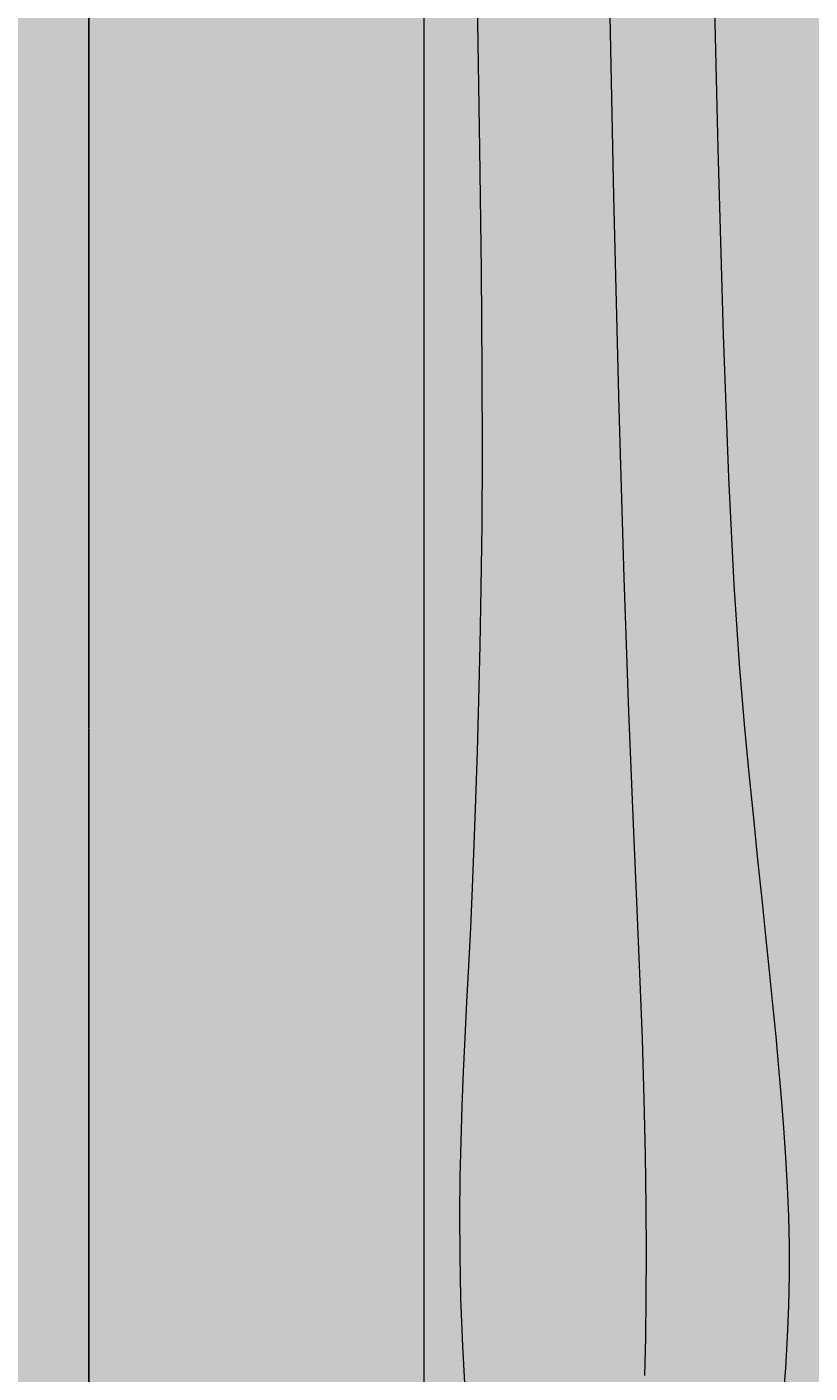
# Model space of a CAD drawing. Units: millimetres. Extents: x -229 to 16545, y -10488 to 4272.
# Tile 16 of 29: x 11804 to 12216, y -3417 to -2708. Entities that reach past the tile are written whole.
import ezdxf

# ---------------------------------------------------------------- set-up
doc = ezdxf.new("R2010")
doc.units = ezdxf.units.MM
for name, color, linetype, lineweight in [('A-ANNO-DIMS', 2, 'Continuous', 18), ('A-FURN', 8, 'Continuous', 18), ('A-FURN-PATT', 252, 'Continuous', 13)]:
    doc.layers.add(name, color=color, linetype=linetype, lineweight=lineweight)
doc.layers.add('A-FLOR-PATT', color=254, linetype='Continuous', lineweight=13, true_color=0xfeeab9)
doc.styles.get("Standard").update_dxf_attribs({"font": 'arial.ttf'})
doc.dimstyles.get("Standard").update_dxf_attribs({"dimtxt": 0.18, "dimasz": 0.18, "dimexe": 0.18, "dimexo": 0.0625, "dimgap": 0.09, "dimtad": 0, "dimtih": 1, "dimtoh": 1, "dimdec": 4, "dimzin": 0, "dimdsep": 46, "dimtxsty": 'Standard', "dimcen": 0.09, "dimadec": 0, "dimazin": 0, "dimtfac": 1, "dimtdec": 4, "dimtofl": 0, "dimtmove": 0, "dimatfit": 3, "dimfxl": 1, "dimtolj": 1, "dimtzin": 0, "dimarcsym": 0})

# ---------------------------------------------------------------- blocks, each defined once
blk = doc.blocks.new('Table - Rectangular Woodgrain 60 x 30 in.')
blk.add_line((0, -30), (60, -30))
for points in [[(8.0098, -22.2501), (14.4094, -22.1011), (19.4168, -21.9535), (23.25, -21.8083), (26.1269, -21.6663), (28.2656, -21.5281), (29.884, -21.3947), (31.2, -21.2667), (32.3967, -21.1448), (33.5172, -21.0292), (34.5697, -20.9198), (35.5625, -20.8167), (36.5037, -20.7198), (37.4015, -20.6292), (38.2642, -20.5448), (39.1, -20.4667), (39.9164, -20.3951), (40.7187, -20.3313), (41.5117, -20.2768), (42.3, -20.2333), (43.0883, -20.2024), (43.8812, -20.1854), (44.6836, -20.1841), (45.5, -20.2), (46.3328, -20.234), (47.1747, -20.2844), (48.0163, -20.3488)], [(8.6355, -25.0504), (15.7026, -24.9031), (21.4049, -24.7606), (25.9458, -24.625), (29.529, -24.4988), (32.3578, -24.3844), (34.6359, -24.284), (36.5667, -24.2), (38.3213, -24.1341), (39.9417, -24.0854), (41.437, -24.0523), (42.8167, -24.0333), (44.0901, -24.0268), (45.2667, -24.0313), (46.3557, -24.0451), (47.3667, -24.0667)], [(10.45, -28.5698), (14.407, -28.5012), (17.675, -28.4584), (20.3711, -28.4374), (22.6125, -28.4344), (24.5164, -28.4455), (26.2, -28.4667), (27.762, -28.4947), (29.2276, -28.5281), (30.6033, -28.5663), (31.8958, -28.6084), (33.1118, -28.6535), (34.2578, -28.7011), (35.3405, -28.7501), (36.3666, -28.8), (37.3443, -28.8497), (38.288, -28.8974), (39.2137, -28.9412), (40.1375, -28.9792), (41.0753, -29.0093), (42.0432, -29.0297), (43.0572, -29.0384), (44.1333, -29.0333), (45.2936, -29.0114), (46.5843, -28.9641), (48.0579, -28.8816)]]:
    blk.add_lwpolyline(points)
blk = doc.blocks.new('*D41')
at = {"layer": 'A-ANNO-DIMS', "color": 0, "lineweight": -2, "transparency": 16777216}
for p, q in [((12012.63, -2489.42), (11836.03, -2489.42)), ((11836.21, -2489.6), (11836.21, -3077.54)), ((11836.21, -3665.84), (11836.21, -3077.9)), ((12012.63, -3666.02), (11836.03, -3666.02))]:
    blk.add_line(p, q, dxfattribs=at)
at = {"layer": 'A-ANNO-DIMS', "color": 0, "transparency": 16777216}
for points in [[(11836.18, -2489.6), (11836.24, -2489.6), (11836.21, -2489.42)], [(11836.18, -3665.84), (11836.24, -3665.84), (11836.21, -3666.02)]]:
    blk.add_solid(points, dxfattribs=at)
at = {"layer": 'Defpoints', "color": 0, "transparency": 16777216}
for p in [(12012.7, -2489.42), (11836.21, -3666.02), (12012.7, -3666.02)]:
    blk.add_point(p, dxfattribs=at)
at = {"layer": 'A-ANNO-DIMS', "color": 0, "transparency": 16777216, "insert": (11836.21, -3077.72), "char_height": 0.18, "attachment_point": 5}
blk.add_mtext('\\A1;LOW TABLE 1177', dxfattribs=at)
blk = doc.blocks.new('*D101')
at = {"layer": 'A-ANNO-DIMS', "color": 0, "lineweight": -2, "transparency": 16777216}
for p, q in [((10907.81, -3049.71), (10907.99, -3049.71)), ((10907.9, -3049.8), (10907.9, -3049.62)), ((15176.85, -3049.71), (13576.18, -3049.71))]:
    blk.add_line(p, q, dxfattribs=at)
at = {"layer": 'A-ANNO-DIMS', "color": 0, "transparency": 16777216}
blk.add_solid([(13576.18, -3049.68), (13576.18, -3049.74), (13576, -3049.71)], dxfattribs=at)
at = {"layer": 'Defpoints', "color": 0, "transparency": 16777216}
for p in [(10907.9, -3049.71), (13576, -3049.71)]:
    blk.add_point(p, dxfattribs=at)
at = {"layer": 'A-ANNO-DIMS', "color": 0, "transparency": 16777216, "insert": (15177.3, -3049.71), "char_height": 0.18, "attachment_point": 5}
blk.add_mtext('\\A1;R2668', dxfattribs=at)
blk = doc.blocks.new('*D102')
at = {"layer": 'A-ANNO-DIMS', "color": 0, "lineweight": -2, "transparency": 16777216}
for p, q in [((11192.83, -3049.71), (11193.01, -3049.71)), ((11192.92, -3049.8), (11192.92, -3049.62)), ((15217.18, -3049.71), (13708.26, -3049.71))]:
    blk.add_line(p, q, dxfattribs=at)
at = {"layer": 'A-ANNO-DIMS', "color": 0, "transparency": 16777216}
blk.add_solid([(13708.26, -3049.68), (13708.26, -3049.74), (13708.08, -3049.71)], dxfattribs=at)
at = {"layer": 'Defpoints', "color": 0, "transparency": 16777216}
for p in [(11192.92, -3049.71), (13708.08, -3049.71)]:
    blk.add_point(p, dxfattribs=at)
at = {"layer": 'A-ANNO-DIMS', "color": 0, "transparency": 16777216, "insert": (15217.62, -3049.71), "char_height": 0.18, "attachment_point": 5}
blk.add_mtext('\\A1;R2515', dxfattribs=at)

msp = doc.modelspace()

# ---------------------------------------------------------------- hatches: boundary and pattern name
at = {"layer": 'A-FLOR-PATT', "transparency": 33554592}
h = msp.add_hatch(color=256, dxfattribs=at)
h.dxf.hatch_style = 1
h.paths.add_polyline_path([(7975.933, -5325.772), (7943.121, -5325.772), (7943.121, -4576.49, 0.4014527), (7225.933, -5325.772, 0.4014527), (6508.746, -4576.49), (6508.746, -5325.772), (6475.933, -5325.772), (6475.933, -5438.272), (5975.933, -5438.272), (5975.933, -7267.724), (5975.933, -7438.272), (6478.619, -7438.272), (6463.448, -7355.919), (6464.88, -7356.837), (6463.849, -7358.097), (6478.619, -7438.272), (6610.327, -7438.272), (6632.656, -7409.564), (6632.525, -7406.967), (6634.208, -7407.569), (6619.273, -7426.77), (6654.466, -7438.272), (7610.517, -7438.272), (7607.41, -7421.409), (7608.842, -7422.327), (7607.812, -7423.587), (7610.517, -7438.272), (7975.933, -7438.272)])
h.paths.add_polyline_path([(13785.933, -1208.272), (9555.933, -1208.272), (9555.933, -961.785), (9705.933, -961.785), (9705.933, -918.035), (10704.976, -918.035, 0.4014527), (9705.933, 38.215), (9555.933, 38.215), (9555.933, 2021.728), (5975.933, 2021.728), (5975.933, 755.492), (5745.933, 755.492), (5745.933, 1427.266), (2918.813, 1427.266), (2918.813, -492.942), (5013.319, -492.942), (5013.319, -978.272), (5745.933, -978.272), (5745.933, -397.513), (5975.933, -397.513), (5975.933, -1208.272), (4560.933, -1208.272), (4560.933, -1265.772), (4448.433, -1265.772), (4448.433, -1298.585), (4445.933, -1298.585), (3699.151, -1298.585, 0.4014527), (4448.433, -2015.772), (4560.933, -2015.772), (4560.933, -2384.177), (5745.933, -2384.177), (5799.402, -2384.177), (5799.402, -4518.272), (5975.933, -4518.272), (5975.933, -5208.272), (6475.933, -5208.272), (6475.933, -4575.772), (6508.746, -4575.772), (6508.746, -4576.49, -0.3564726), (7216.672, -5208.272), (7235.194, -5208.272, -0.3564726), (7943.121, -4576.49), (7943.121, -4575.772), (7975.933, -4575.772), (7975.933, -5208.272), (11176.247, -5208.272), (11159.44, -5191.465), (10520.768, -5191.465), (10520.768, -4888.936), (10571.19, -4888.936), (10571.19, -4872.129), (10772.876, -4872.129), (10772.876, -4888.936), (10789.683, -4888.936), (10789.683, -4872.129), (10991.368, -4872.129), (10991.368, -4888.936), (11041.79, -4888.936), (11041.79, -4872.129), (11058.597, -4872.129, -0.0909091), (11428.354, -4872.129), (11445.162, -4872.129), (11445.162, -4888.936), (11529.197, -4888.936), (11529.197, -5191.465), (11327.512, -5191.465), (11310.704, -5208.272), (13785.933, -5208.272)])
h.paths.add_polyline_path([(11047.216, -1630.944, -1), (11402.816, -1630.944, -1)], flags=16)
h.paths.add_polyline_path([(11148.816, -1630.944), (11225.016, -1554.744), (11301.216, -1630.944), (11225.016, -1707.144)], flags=0)
h.paths.add_polyline_path([(11199.616, -1630.944, -1), (11250.416, -1630.944, -1)], flags=0)
h.paths.add_polyline_path([(11588.751, -2096.259), (11588.751, -1543.254, -0.266667), (12864.918, -1543.254), (12864.918, -2096.259), (12737.302, -2096.259), (12737.302, -2063.121), (11716.368, -2063.121), (11716.368, -2096.259)], flags=16)
h.paths.add_polyline_path([(12012.696, -2489.42), (12600.997, -2489.42), (12600.997, -3666.022), (12012.696, -3666.022)], flags=16)
h.paths.add_polyline_path([(12176.41, -3599.403), (12174.938, -3609.076), (12173.789, -3618.819), (12173.09, -3628.559), (12172.973, -3638.221), (12173.89, -3652.852), (12175.008, -3657.025), (12172.909, -3643.473), (12173.142, -3624.297), (12175.386, -3605.273)], flags=0)
h.paths.add_polyline_path([(8026.289, -286.944), (7737.703, -287.19), (7734.87, -269.156), (8029.092, -268.905)], flags=16)
h.paths.add_polyline_path([(7733.453, -260.139), (7710.784, -115.865), (7557.191, -115.996), (7556.999, 109.744), (7412.687, 132.166), (7412.433, 429.206), (7556.707, 451.876), (7556.568, 614.769), (7412.256, 637.19), (7412.003, 934.231), (7556.276, 956.9), (7556.084, 1182.639), (7709.677, 1182.77), (7732.099, 1327.082), (8029.14, 1327.335), (8051.808, 1183.062), (8205.401, 1183.192), (8205.594, 957.454), (8349.906, 935.031), (8350.159, 637.99), (8205.885, 615.322), (8206.024, 452.43), (8350.336, 430.006), (8350.59, 132.965), (8206.316, 110.298), (8206.509, -115.442), (8052.916, -115.573), (8030.493, -259.885)], flags=16)
h.paths.add_polyline_path([(12261.416, -3475.554), (12262.632, -3486.776), (12264.032, -3497.007), (12265.554, -3506.365), (12267.136, -3514.968), (12268.719, -3522.935), (12271.304, -3535.59), (12273.606, -3548.078), (12275.271, -3561.064), (12275.93, -3574.938), (12275.325, -3590.3), (12273.425, -3607.964), (12270.795, -3625.658), (12268.066, -3641.063), (12266.318, -3649.679), (12265.456, -3653.626), (12263.984, -3659.846), (12264.032, -3659.566), (12264.342, -3658.241), (12264.807, -3656.37), (12265.456, -3653.626), (12266.318, -3649.679), (12267.409, -3644.302), (12268.668, -3637.664), (12270.019, -3630.037), (12271.384, -3621.695), (12272.69, -3612.908), (12273.857, -3603.948), (12274.81, -3595.088), (12275.47, -3586.601), (12275.782, -3578.689), (12275.757, -3571.292), (12275.423, -3564.275), (12274.816, -3557.512), (12273.964, -3550.872), (12272.896, -3544.224), (12271.645, -3537.439), (12270.24, -3530.385), (12267.543, -3517.181), (12264.612, -3501.247), (12261.849, -3481.059)], flags=0)
h.paths.add_polyline_path([(12332.136, -3408.03), (12333.483, -3416.79), (12335.077, -3424.54), (12336.915, -3431.355), (12338.991, -3437.32), (12341.266, -3442.55), (12343.694, -3447.166), (12346.229, -3451.292), (12348.826, -3455.051), (12351.438, -3458.563), (12357.476, -3466.491), (12363.61, -3476.575), (12368.309, -3489.762), (12369.929, -3503.427), (12369.842, -3516.511), (12368.43, -3530.867), (12365.816, -3545.835), (12362.382, -3559.786), (12360.968, -3564.487), (12363.063, -3557.021), (12364.898, -3549.566), (12366.473, -3542.077), (12367.773, -3534.631), (12368.781, -3527.301), (12369.483, -3520.162), (12369.863, -3513.291), (12369.906, -3506.759), (12369.599, -3500.643), (12368.93, -3494.999), (12367.924, -3489.796), (12366.61, -3484.994), (12365.024, -3480.542), (12363.19, -3476.399), (12361.141, -3472.516), (12358.909, -3468.847), (12356.525, -3465.347), (12354.02, -3461.954), (12351.438, -3458.563), (12345.462, -3450.529), (12339.923, -3439.996), (12335.85, -3428.296), (12332.68, -3412.888)], flags=0)
h.paths.add_polyline_path([(12385.287, -3334.612), (12384.977, -3342.409), (12385.02, -3349.196), (12385.4, -3355.066), (12386.104, -3360.105), (12387.112, -3364.41), (12388.412, -3368.071), (12389.987, -3371.181), (12391.823, -3373.832), (12393.919, -3376.097), (12396.337, -3377.978), (12399.153, -3379.462), (12402.445, -3380.531), (12406.289, -3381.172), (12410.758, -3381.371), (12415.935, -3381.106), (12421.893, -3380.368), (12428.658, -3379.159), (12436.069, -3377.55), (12443.907, -3375.635), (12451.961, -3373.505), (12460.015, -3371.254), (12467.853, -3368.971), (12475.263, -3366.749), (12482.029, -3364.68), (12491.877, -3361.657), (12497.701, -3360.107), (12501.639, -3359.288), (12510.135, -3358.326), (12519.662, -3365.412), (12524.243, -3378.911), (12523.764, -3390.7), (12520.746, -3401.577), (12514.248, -3415.634), (12511.518, -3420.418), (12515.856, -3412.154), (12519.153, -3405.024), (12521.516, -3398.804), (12523.049, -3393.276), (12523.865, -3388.212), (12524.059, -3383.441), (12523.7, -3378.958), (12522.853, -3374.815), (12521.576, -3371.054), (12519.931, -3367.722), (12517.982, -3364.865), (12515.786, -3362.529), (12513.405, -3360.758), (12510.877, -3359.588), (12508.136, -3358.982), (12505.086, -3358.897), (12501.639, -3359.288), (12497.701, -3360.107), (12493.183, -3361.309), (12487.988, -3362.851), (12476.403, -3366.408), (12463.335, -3370.326), (12447.372, -3374.788), (12431.759, -3378.604), (12418.504, -3380.974), (12405.811, -3381.624), (12394.725, -3378.025), (12388.039, -3368.367), (12385.583, -3357.877), (12384.826, -3346.204), (12385.428, -3331.059), (12385.953, -3325.719)], flags=0)
h.paths.add_polyline_path([(7880.016, 1173.969), (7880.373, 1175.495), (7880.433, 1175.851), (7879.484, 1171.818)], flags=0)
h.paths.add_polyline_path([(7802.33, 874.962), (7800.771, 885.032), (7798.932, 893.941), (7796.811, 901.774), (7794.419, 908.63), (7791.798, 914.639), (7789.002, 919.945), (7786.083, 924.686), (7783.093, 929.005), (7780.087, 933.043), (7774.996, 939.717), (7768.406, 949.37), (7762.174, 963.427), (7759.342, 978.002), (7758.629, 991.888), (7759.492, 1007.928), (7761.801, 1025.496), (7765.392, 1044.035), (7766.625, 1049.048), (7764.522, 1039.543), (7762.719, 1030.232), (7761.232, 1021.168), (7760.08, 1012.405), (7759.28, 1003.994), (7758.849, 995.988), (7758.806, 988.44), (7759.167, 981.404), (7759.942, 974.914), (7761.104, 968.936), (7762.617, 963.414), (7764.448, 958.299), (7766.559, 953.535), (7768.918, 949.073), (7771.487, 944.856), (7774.232, 940.835), (7777.115, 936.938), (7782.377, 930.041), (7787.845, 922.139), (7793.348, 911.698), (7798.042, 898.247), (7801.702, 880.527)], flags=0)
h.paths.add_polyline_path([(12519.068, -3228.534), (12519.615, -3236.235), (12520.529, -3242.343), (12521.78, -3247.103), (12523.337, -3250.758), (12525.171, -3253.556), (12527.248, -3255.709), (12529.522, -3257.296), (12531.95, -3258.361), (12534.486, -3258.949), (12537.082, -3259.11), (12539.694, -3258.888), (12542.277, -3258.329), (12544.781, -3257.478), (12547.173, -3256.388), (12549.46, -3255.129), (12550.455, -3254.517), (12555.825, -3251.109), (12557.835, -3249.942), (12565.181, -3246.404), (12574.565, -3253.032), (12576.931, -3265.022), (12576.627, -3277.425), (12575.416, -3290.819), (12574.851, -3295.392), (12575.708, -3287.593), (12576.322, -3280.806), (12576.688, -3274.939), (12576.812, -3269.899), (12576.688, -3265.593), (12576.322, -3261.932), (12575.708, -3258.822), (12574.851, -3256.172), (12573.753, -3253.905), (12572.439, -3252.005), (12570.943, -3250.474), (12569.293, -3249.309), (12567.523, -3248.513), (12565.658, -3248.083), (12563.732, -3248.022), (12561.777, -3248.328), (12559.814, -3248.989), (12557.835, -3249.942), (12555.825, -3251.109), (12553.77, -3252.413), (12551.652, -3253.78), (12549.46, -3255.129), (12543.167, -3258.594), (12532.661, -3259.485), (12524.685, -3253.923), (12520.949, -3245.152), (12519.138, -3233.042)], flags=0)
h.paths.add_polyline_path([(7741.293, 790.501), (7741.641, 799.467), (7741.584, 807.269), (7741.141, 814.015), (7740.329, 819.809), (7739.165, 824.757), (7737.667, 828.966), (7735.853, 832.541), (7733.74, 835.586), (7731.348, 838.188), (7728.71, 840.348), (7725.861, 842.052), (7722.836, 843.28), (7719.671, 844.015), (7716.4, 844.237), (7713.06, 843.932), (7709.684, 843.081), (7706.304, 841.686), (7702.923, 839.834), (7699.543, 837.629), (7696.164, 835.178), (7692.784, 832.585), (7684.718, 826.315), (7675.609, 820.63), (7664.001, 817.274), (7654.105, 821.884), (7647.171, 832.02), (7644.191, 846.522), (7646.321, 860.288), (7647.49, 864.223), (7645.946, 857.865), (7645.046, 852.044), (7644.827, 846.557), (7645.243, 841.404), (7646.221, 836.642), (7647.693, 832.318), (7649.587, 828.489), (7651.832, 825.206), (7654.359, 822.523), (7657.097, 820.49), (7659.984, 819.145), (7662.993, 818.452), (7666.108, 818.357), (7669.311, 818.809), (7672.583, 819.755), (7675.908, 821.139), (7679.268, 822.913), (7682.645, 825.021), (7686.025, 827.401), (7689.404, 829.958), (7692.784, 832.585), (7700.505, 838.509), (7709.871, 843.64), (7721.436, 844.698), (7733.277, 837.617), (7739.571, 825.214), (7741.557, 811.049), (7741.669, 795.575)], flags=0)
h.paths.add_polyline_path([(8377.641, 137.216), (8359.607, 134.382), (8359.356, 428.605), (8377.395, 425.802)], flags=16)
h.paths.add_polyline_path([(7650.715, 668.465), (7650.08, 677.319), (7649.023, 684.34), (7647.579, 689.811), (7645.785, 694.012), (7643.675, 697.228), (7641.286, 699.7), (7638.669, 701.521), (7635.876, 702.744), (7632.96, 703.419), (7629.974, 703.601), (7626.971, 703.344), (7624.004, 702.697), (7621.125, 701.717), (7618.375, 700.462), (7615.749, 699.013), (7614.561, 698.279), (7608.435, 694.382), (7606.125, 693.04), (7598.981, 689.594), (7589.669, 693.773), (7585.26, 702.856), (7584.221, 713.11), (7584.49, 724.584), (7585.863, 739.937), (7586.518, 745.277), (7585.539, 736.31), (7584.841, 728.507), (7584.424, 721.761), (7584.288, 715.966), (7584.433, 711.016), (7584.86, 706.807), (7585.567, 703.231), (7586.556, 700.186), (7587.821, 697.58), (7589.332, 695.397), (7591.053, 693.637), (7592.951, 692.3), (7594.989, 691.385), (7597.132, 690.895), (7599.346, 690.826), (7601.594, 691.18), (7603.851, 691.943), (7606.125, 693.04), (7608.435, 694.382), (7610.797, 695.885), (7613.229, 697.458), (7620.475, 701.929), (7632.001, 704.44), (7643.476, 699.417), (7648.536, 687.571), (7650.63, 673.661)], flags=0)
h.paths.add_polyline_path([(7385.628, 136.37), (7385.382, 424.956), (7403.416, 427.789), (7403.667, 133.567)], flags=16)
h.paths.add_polyline_path([(12993.884, -2257.186), (12959.588, -2257.186), (12959.588, -2125.099), (13531.966, -2125.099, -0.1904762), (13531.966, -3974.321), (12959.588, -3974.321), (12959.588, -3842.233), (12993.884, -3842.233)], flags=16)
h.paths.add_polyline_path([(13413.486, -3313.884), (13413.486, -2785.535), (13562.885, -2785.535, -0.0496282), (13562.885, -3313.884)], flags=0)
h.paths.add_polyline_path([(8377.21, 642.241), (8359.176, 639.407), (8358.925, 933.629), (8376.964, 930.826)], flags=16)
h.paths.add_polyline_path([(13086.058, -1864.83), (13086.058, -1449.84), (13501.048, -1449.84), (13501.048, -1864.83)], flags=16)
h.paths.add_polyline_path([(13305.814, -1862.197), (13302.103, -1859.624), (13298.088, -1857.068), (13293.799, -1854.536), (13289.262, -1852.031), (13284.504, -1849.559), (13279.554, -1847.125), (13274.439, -1844.735), (13269.17, -1842.389), (13263.701, -1840.081), (13257.97, -1837.797), (13251.914, -1835.525), (13245.472, -1833.252), (13238.582, -1830.968), (13231.18, -1828.66), (13223.206, -1826.315), (13209.182, -1822.458), (13204.584, -1821.48), (13217.962, -1824.773), (13235.072, -1829.804), (13248.777, -1834.349), (13260.829, -1838.869), (13274.479, -1844.63), (13289.675, -1852.101), (13302.553, -1859.704)], flags=0)
h.paths.add_polyline_path([(13428.104, -1820.994), (13419.007, -1818.141), (13409.95, -1815.4), (13400.766, -1812.747), (13391.271, -1810.151), (13376.087, -1806.251), (13370.618, -1805.019), (13386.304, -1808.794), (13405.087, -1813.928), (13423.014, -1819.354)], flags=0)
h.paths.add_polyline_path([(7385.197, 641.395), (7384.951, 929.98), (7402.986, 932.814), (7403.236, 638.592)], flags=16)
h.paths.add_polyline_path([(13262.537, -1725.526), (13253.246, -1724.74), (13244.516, -1724.117), (13235.94, -1723.625), (13223.267, -1723.062), (13217.598, -1722.912), (13231.966, -1723.397), (13248.733, -1724.359), (13266.899, -1725.895), (13272.802, -1726.502)], flags=0)
h.paths.add_polyline_path([(13191.893, -1641.137), (13208.675, -1640.506), (13214.057, -1640.258), (13197.763, -1640.936)], flags=0)
h.paths.add_polyline_path([(13097.524, -1608.457), (13114.284, -1609.031), (13120.126, -1609.105), (13103.045, -1608.71)], flags=0)
h.paths.add_polyline_path([(13465.328, -1521.577), (13473.906, -1517.015), (13481.761, -1511.636), (13492.562, -1502.076), (13495.327, -1497.933), (13485.818, -1508.858), (13470.208, -1519.547)], flags=0)
h.paths.add_polyline_path([(13175.015, -1500.891), (13184.046, -1501.807), (13192.721, -1502.52), (13201.114, -1503.034), (13209.273, -1503.351), (13217.244, -1503.476), (13225.078, -1503.41), (13232.821, -1503.16), (13240.524, -1502.728), (13248.233, -1502.117), (13255.993, -1501.322), (13263.825, -1500.293), (13271.746, -1498.974), (13279.775, -1497.305), (13287.928, -1495.229), (13296.222, -1492.688), (13304.675, -1489.622), (13313.304, -1485.975), (13322.089, -1481.727), (13330.859, -1477.028), (13339.408, -1472.063), (13347.526, -1467.02), (13355.006, -1462.087), (13364.86, -1455.202), (13367.224, -1453.299), (13358.544, -1459.754), (13343.348, -1469.775), (13326.143, -1479.767), (13309.023, -1488.045), (13292.249, -1494.129), (13276.009, -1498.264), (13260.299, -1500.88), (13244.401, -1502.51), (13228.945, -1503.378), (13213.316, -1503.508), (13197.047, -1502.876), (13180.088, -1501.481)], flags=0)
h.paths.add_polyline_path([(7733.501, 1336.101), (7736.303, 1354.14), (8024.889, 1354.386), (8027.723, 1336.352)], flags=16)
at = {"layer": 'A-FURN-PATT', "transparency": 33554569}
h = msp.add_hatch(color=256, dxfattribs=at)
h.dxf.hatch_style = 1
h.paths.add_polyline_path([(12600.997, -2489.42), (12553.933, -2489.42), (12553.58, -2583.852), (12552.584, -2666.503), (12551.036, -2738.644), (12549.03, -2801.547), (12546.656, -2856.483), (12544.004, -2904.723), (12541.171, -2947.542), (12538.245, -2986.207), (12535.313, -3021.787), (12532.444, -3054.526), (12529.695, -3084.461), (12527.132, -3111.629), (12524.814, -3136.073), (12522.802, -3157.826), (12521.157, -3176.928), (12519.941, -3193.42), (12519.202, -3207.371), (12518.921, -3218.994), (12519.068, -3228.534), (12519.615, -3236.235), (12520.529, -3242.343), (12521.78, -3247.103), (12523.337, -3250.758), (12525.171, -3253.556), (12527.248, -3255.709), (12529.522, -3257.296), (12531.95, -3258.361), (12534.486, -3258.949), (12537.082, -3259.11), (12539.694, -3258.888), (12542.277, -3258.329), (12544.781, -3257.478), (12547.173, -3256.388), (12549.46, -3255.129), (12551.652, -3253.78), (12559.563, -3248.675), (12566.794, -3247.543), (12572.687, -3251.706), (12575.978, -3258.498), (12576.872, -3267.431), (12576.627, -3277.425), (12575.708, -3287.593), (12574.851, -3295.392), (12573.749, -3304.309), (12572.419, -3314.522), (12570.874, -3326.221), (12569.131, -3339.597), (12567.203, -3354.842), (12565.107, -3372.146), (12562.857, -3391.705), (12560.469, -3413.705), (12557.959, -3438.275), (12555.343, -3465.264), (12552.633, -3494.46), (12549.848, -3525.645), (12547.001, -3558.61), (12544.106, -3593.137), (12541.184, -3629.012), (12538.245, -3666.022), (12600.997, -3666.022)])
h.paths.add_polyline_path([(12544.004, -2904.723), (12546.656, -2856.483), (12549.03, -2801.547), (12551.036, -2738.644), (12552.584, -2666.503), (12553.58, -2583.852), (12553.933, -2489.42), (12420.585, -2489.42), (12422.824, -2618.374), (12423.791, -2723.534), (12423.687, -2808.136), (12422.708, -2875.41), (12421.057, -2928.591), (12418.93, -2970.907), (12416.527, -3005.595), (12414.049, -3035.885), (12411.656, -3064.467), (12409.37, -3091.846), (12407.177, -3117.984), (12405.059, -3142.842), (12403.004, -3166.384), (12400.994, -3188.569), (12399.016, -3209.359), (12397.053, -3228.718), (12395.1, -3246.62), (12393.191, -3263.097), (12391.376, -3278.194), (12389.699, -3291.961), (12388.205, -3304.438), (12386.942, -3315.677), (12385.953, -3325.719), (12385.287, -3334.612), (12384.977, -3342.409), (12385.02, -3349.196), (12385.4, -3355.066), (12386.104, -3360.105), (12387.112, -3364.41), (12388.412, -3368.071), (12389.987, -3371.181), (12391.823, -3373.832), (12393.919, -3376.097), (12396.337, -3377.978), (12399.153, -3379.462), (12402.445, -3380.531), (12406.289, -3381.172), (12410.758, -3381.371), (12415.935, -3381.106), (12421.893, -3380.368), (12428.658, -3379.159), (12436.069, -3377.55), (12443.907, -3375.635), (12451.961, -3373.505), (12460.015, -3371.254), (12467.853, -3368.971), (12475.263, -3366.749), (12482.029, -3364.68), (12491.877, -3361.657), (12502.516, -3358.826), (12511.128, -3359.064), (12517.01, -3363.44), (12520.955, -3369.223), (12523.527, -3376.802), (12524.25, -3385.824), (12522.632, -3395.865), (12519.153, -3405.024), (12515.856, -3412.154), (12511.518, -3420.418), (12506.031, -3430.037), (12499.288, -3441.236), (12491.181, -3454.234), (12481.682, -3469.286), (12471.081, -3486.774), (12459.744, -3507.112), (12448.039, -3530.713), (12436.334, -3557.99), (12424.997, -3589.358), (12414.396, -3625.231), (12404.897, -3666.022), (12538.245, -3666.022), (12541.184, -3629.012), (12544.106, -3593.137), (12547.001, -3558.61), (12549.848, -3525.645), (12552.633, -3494.46), (12555.343, -3465.264), (12557.959, -3438.275), (12560.469, -3413.705), (12562.857, -3391.705), (12565.107, -3372.146), (12567.203, -3354.842), (12569.131, -3339.597), (12570.874, -3326.221), (12572.419, -3314.522), (12573.749, -3304.309), (12574.851, -3295.392), (12575.708, -3287.593), (12576.322, -3280.806), (12576.688, -3274.939), (12576.812, -3269.899), (12576.688, -3265.593), (12576.322, -3261.932), (12575.708, -3258.822), (12574.851, -3256.172), (12573.753, -3253.905), (12572.439, -3252.005), (12570.943, -3250.474), (12569.293, -3249.309), (12567.523, -3248.513), (12565.658, -3248.083), (12563.732, -3248.022), (12561.777, -3248.328), (12559.814, -3248.989), (12557.835, -3249.942), (12555.825, -3251.109), (12553.77, -3252.413), (12547.19, -3256.659), (12539.533, -3259.262), (12531.64, -3258.773), (12524.685, -3253.923), (12520.949, -3245.152), (12519.615, -3236.235), (12519.068, -3228.534), (12518.921, -3218.994), (12519.202, -3207.371), (12519.941, -3193.42), (12521.157, -3176.928), (12522.802, -3157.826), (12524.814, -3136.073), (12527.132, -3111.629), (12529.695, -3084.461), (12532.444, -3054.526), (12535.313, -3021.787), (12538.245, -2986.207), (12541.171, -2947.542)])
h.paths.add_polyline_path([(12418.93, -2970.907), (12421.057, -2928.591), (12422.708, -2875.41), (12423.687, -2808.136), (12423.791, -2723.534), (12422.824, -2618.374), (12420.585, -2489.42), (12349.989, -2489.42), (12347.396, -2591.092), (12345.433, -2678.094), (12343.99, -2752.122), (12342.962, -2814.864), (12342.239, -2868.017), (12341.715, -2913.271), (12341.284, -2952.323), (12340.837, -2986.86), (12340.288, -3018.358), (12339.633, -3047.386), (12338.883, -3074.301), (12338.06, -3099.455), (12337.173, -3123.199), (12336.242, -3145.885), (12335.279, -3167.868), (12334.301, -3189.498), (12333.326, -3211.038), (12332.381, -3232.395), (12331.496, -3253.384), (12330.706, -3273.821), (12330.037, -3293.523), (12329.52, -3312.306), (12329.188, -3329.984), (12329.071, -3346.378), (12329.194, -3361.343), (12329.561, -3374.915), (12330.175, -3387.169), (12331.032, -3398.18), (12332.136, -3408.03), (12333.483, -3416.79), (12335.077, -3424.54), (12336.915, -3431.355), (12338.991, -3437.32), (12341.266, -3442.55), (12343.694, -3447.166), (12346.229, -3451.292), (12348.826, -3455.051), (12351.438, -3458.563), (12357.476, -3466.491), (12362.356, -3474.514), (12365.989, -3482.725), (12368.611, -3492.308), (12369.929, -3503.427), (12369.863, -3513.291), (12369.483, -3520.162), (12368.781, -3527.301), (12367.773, -3534.631), (12366.473, -3542.077), (12364.898, -3549.566), (12363.063, -3557.021), (12360.968, -3564.487), (12358.568, -3572.468), (12355.799, -3581.585), (12352.603, -3592.463), (12348.916, -3605.723), (12344.678, -3621.988), (12339.827, -3641.88), (12334.301, -3666.022), (12404.897, -3666.022), (12414.396, -3625.231), (12424.997, -3589.358), (12436.334, -3557.99), (12448.039, -3530.713), (12459.744, -3507.112), (12471.081, -3486.774), (12481.682, -3469.286), (12491.181, -3454.234), (12499.288, -3441.236), (12506.031, -3430.037), (12511.518, -3420.418), (12515.856, -3412.154), (12519.153, -3405.024), (12521.516, -3398.804), (12523.049, -3393.276), (12523.865, -3388.212), (12524.059, -3383.441), (12523.7, -3378.958), (12522.853, -3374.815), (12521.576, -3371.054), (12519.931, -3367.722), (12517.982, -3364.865), (12515.786, -3362.529), (12513.405, -3360.758), (12510.877, -3359.588), (12508.136, -3358.982), (12505.086, -3358.897), (12501.639, -3359.288), (12497.701, -3360.107), (12493.183, -3361.309), (12487.988, -3362.851), (12476.403, -3366.408), (12463.335, -3370.326), (12451.961, -3373.505), (12439.372, -3376.834), (12424.661, -3380.026), (12412.995, -3381.47), (12402.039, -3380.984), (12393.748, -3376.613), (12389.022, -3369.787), (12386.442, -3362.522), (12385.041, -3352.492), (12384.977, -3342.409), (12385.287, -3334.612), (12385.953, -3325.719), (12386.942, -3315.677), (12388.205, -3304.438), (12389.699, -3291.961), (12391.376, -3278.194), (12393.191, -3263.097), (12395.1, -3246.62), (12397.053, -3228.718), (12399.016, -3209.359), (12400.994, -3188.569), (12403.004, -3166.384), (12405.059, -3142.842), (12407.177, -3117.984), (12409.37, -3091.846), (12411.656, -3064.467), (12414.049, -3035.885), (12416.527, -3005.595)])
h.paths.add_polyline_path([(12340.837, -2986.86), (12341.284, -2952.323), (12341.715, -2913.271), (12342.239, -2868.017), (12342.962, -2814.864), (12343.99, -2752.122), (12345.433, -2678.094), (12347.396, -2591.092), (12349.989, -2489.42), (12248.016, -2489.42), (12253.364, -2589.902), (12257.71, -2678.871), (12261.149, -2757.499), (12263.787, -2826.958), (12265.718, -2888.42), (12267.044, -2943.055), (12267.866, -2992.039), (12268.279, -3036.54), (12268.378, -3077.58), (12268.209, -3115.572), (12267.809, -3150.776), (12267.219, -3183.452), (12266.473, -3213.86), (12265.614, -3242.261), (12264.679, -3268.917), (12263.704, -3294.084), (12262.732, -3317.981), (12261.804, -3340.639), (12260.969, -3362.039), (12260.273, -3382.167), (12259.759, -3401.008), (12259.477, -3418.547), (12259.469, -3434.769), (12259.782, -3449.659), (12260.445, -3463.221), (12261.416, -3475.554), (12262.632, -3486.776), (12264.032, -3497.007), (12265.554, -3506.365), (12267.136, -3514.968), (12268.719, -3522.935), (12271.304, -3535.59), (12273.606, -3548.078), (12275.271, -3561.064), (12275.757, -3571.292), (12275.782, -3578.689), (12275.47, -3586.601), (12274.81, -3595.088), (12273.857, -3603.948), (12272.69, -3612.908), (12271.384, -3621.695), (12270.019, -3630.037), (12268.066, -3641.063), (12265.651, -3652.97), (12264.342, -3658.241), (12264.032, -3659.566), (12263.842, -3660.678), (12263.746, -3661.906), (12263.708, -3663.576), (12263.704, -3666.022), (12334.301, -3666.022), (12339.827, -3641.88), (12344.678, -3621.988), (12348.916, -3605.723), (12352.603, -3592.463), (12355.799, -3581.585), (12358.568, -3572.468), (12360.968, -3564.487), (12363.063, -3557.021), (12364.898, -3549.566), (12366.473, -3542.077), (12367.773, -3534.631), (12368.781, -3527.301), (12369.483, -3520.162), (12369.863, -3513.291), (12369.906, -3506.759), (12369.599, -3500.643), (12368.93, -3494.999), (12367.924, -3489.796), (12366.61, -3484.994), (12365.024, -3480.542), (12363.19, -3476.399), (12361.141, -3472.516), (12358.909, -3468.847), (12356.525, -3465.347), (12354.02, -3461.954), (12347.609, -3453.536), (12342.257, -3444.828), (12337.759, -3434.488), (12335.077, -3424.54), (12333.483, -3416.79), (12332.136, -3408.03), (12331.032, -3398.18), (12330.175, -3387.169), (12329.561, -3374.915), (12329.194, -3361.343), (12329.071, -3346.378), (12329.188, -3329.984), (12329.52, -3312.306), (12330.037, -3293.523), (12330.706, -3273.821), (12331.496, -3253.384), (12332.381, -3232.395), (12333.326, -3211.038), (12334.301, -3189.498), (12335.279, -3167.868), (12336.242, -3145.885), (12337.173, -3123.199), (12338.06, -3099.455), (12338.883, -3074.301), (12339.633, -3047.386), (12340.288, -3018.358)])
h.paths.add_polyline_path([(12267.866, -2992.039), (12267.044, -2943.055), (12265.718, -2888.42), (12263.787, -2826.958), (12261.149, -2757.499), (12257.71, -2678.871), (12253.364, -2589.902), (12248.016, -2489.42), (12161.732, -2489.42), (12164.672, -2646.493), (12167.594, -2771.989), (12170.488, -2870.184), (12173.336, -2945.353), (12176.12, -3001.769), (12178.83, -3043.709), (12181.446, -3075.446), (12183.956, -3101.253), (12186.347, -3124.72), (12188.614, -3146.693), (12190.759, -3167.333), (12192.781, -3186.802), (12194.681, -3205.259), (12196.458, -3222.865), (12198.113, -3239.782), (12199.644, -3256.172), (12201.048, -3272.182), (12202.3, -3287.915), (12203.368, -3303.466), (12204.221, -3318.924), (12204.827, -3334.383), (12205.161, -3349.932), (12205.186, -3365.667), (12204.874, -3381.676), (12204.208, -3398.008), (12203.219, -3414.517), (12201.956, -3431.021), (12200.462, -3447.329), (12198.784, -3463.254), (12196.97, -3478.607), (12195.062, -3493.203), (12193.108, -3506.853), (12191.149, -3519.429), (12189.196, -3531.038), (12187.259, -3541.853), (12185.347, -3552.039), (12183.462, -3561.763), (12181.619, -3571.2), (12179.819, -3580.51), (12178.073, -3589.87), (12176.41, -3599.403), (12174.938, -3609.076), (12173.789, -3618.819), (12173.09, -3628.559), (12172.973, -3638.221), (12173.569, -3647.734), (12175.008, -3657.025), (12177.42, -3666.022), (12263.654, -3666.022), (12263.777, -3660.515), (12264.807, -3656.37), (12265.456, -3653.626), (12266.318, -3649.679), (12267.409, -3644.302), (12268.668, -3637.664), (12270.019, -3630.037), (12271.384, -3621.695), (12272.69, -3612.908), (12273.857, -3603.948), (12274.81, -3595.088), (12275.47, -3586.601), (12275.782, -3578.689), (12275.757, -3571.292), (12275.423, -3564.275), (12274.816, -3557.512), (12273.964, -3550.872), (12272.896, -3544.224), (12271.645, -3537.439), (12270.24, -3530.385), (12267.543, -3517.181), (12265.554, -3506.365), (12264.032, -3497.007), (12262.632, -3486.776), (12261.416, -3475.554), (12260.445, -3463.221), (12259.782, -3449.659), (12259.469, -3434.769), (12259.477, -3418.547), (12259.759, -3401.008), (12260.273, -3382.167), (12260.969, -3362.039), (12261.804, -3340.639), (12262.732, -3317.981), (12263.704, -3294.084), (12264.679, -3268.917), (12265.614, -3242.261), (12266.473, -3213.86), (12267.219, -3183.452), (12267.809, -3150.776), (12268.209, -3115.572), (12268.378, -3077.58), (12268.279, -3036.54)])
h.paths.add_polyline_path([(12178.83, -3043.709), (12176.12, -3001.769), (12173.336, -2945.353), (12170.488, -2870.184), (12167.594, -2771.989), (12164.672, -2646.493), (12161.732, -2489.42), (12106.824, -2489.42), (12109.758, -2658.763), (12112.646, -2797.349), (12115.441, -2909.171), (12118.1, -2998.218), (12120.575, -3068.485), (12122.818, -3123.958), (12124.787, -3168.631), (12126.434, -3206.494), (12127.727, -3240.902), (12128.682, -3272.678), (12129.331, -3302.001), (12129.703, -3329.057), (12129.831, -3354.028), (12129.742, -3377.101), (12129.472, -3398.457), (12129.048, -3418.282), (12128.499, -3436.761), (12127.832, -3454.092), (12127.062, -3470.478), (12126.189, -3486.119), (12125.224, -3501.217), (12124.177, -3515.972), (12123.052, -3530.585), (12121.857, -3545.257), (12120.61, -3560.145), (12119.355, -3575.225), (12118.147, -3590.433), (12117.037, -3605.699), (12116.082, -3620.96), (12115.331, -3636.144), (12114.843, -3651.187), (12114.668, -3666.022), (12177.42, -3666.022), (12175.008, -3657.025), (12173.569, -3647.734), (12172.973, -3638.221), (12173.09, -3628.559), (12173.789, -3618.819), (12174.938, -3609.076), (12176.41, -3599.403), (12178.073, -3589.87), (12179.819, -3580.51), (12181.619, -3571.2), (12183.462, -3561.763), (12185.347, -3552.039), (12187.259, -3541.853), (12189.196, -3531.038), (12191.149, -3519.429), (12193.108, -3506.853), (12195.062, -3493.203), (12196.97, -3478.607), (12198.784, -3463.254), (12200.462, -3447.329), (12201.956, -3431.021), (12203.219, -3414.517), (12204.208, -3398.008), (12204.874, -3381.676), (12205.186, -3365.667), (12205.161, -3349.932), (12204.827, -3334.383), (12204.221, -3318.924), (12203.368, -3303.466), (12202.3, -3287.915), (12201.048, -3272.182), (12199.644, -3256.172), (12198.113, -3239.782), (12196.458, -3222.865), (12194.681, -3205.259), (12192.781, -3186.802), (12190.759, -3167.333), (12188.614, -3146.693), (12186.347, -3124.72), (12183.956, -3101.253), (12181.446, -3075.446)])
h.paths.add_polyline_path([(12120.575, -3068.485), (12118.1, -2998.218), (12115.441, -2909.171), (12112.646, -2797.349), (12109.758, -2658.763), (12106.824, -2489.42), (12036.228, -2489.42), (12038.815, -2600.936), (12040.742, -2694.345), (12042.088, -2771.942), (12042.927, -2836.027), (12043.339, -2888.898), (12043.398, -2932.852), (12043.18, -2970.187), (12042.764, -3003.203), (12042.215, -3033.834), (12041.56, -3062.574), (12040.811, -3089.552), (12039.985, -3114.898), (12039.101, -3138.743), (12038.168, -3161.217), (12037.207, -3182.448), (12036.228, -3202.57), (12035.254, -3221.743), (12034.318, -3240.249), (12033.459, -3258.402), (12032.714, -3276.518), (12032.124, -3294.908), (12031.724, -3313.888), (12031.553, -3333.773), (12031.653, -3354.875), (12032.083, -3377.629), (12033.01, -3402.94), (12034.628, -3431.837), (12037.126, -3465.345), (12040.697, -3504.492), (12045.533, -3550.301), (12051.822, -3603.803), (12059.76, -3666.022), (12114.668, -3666.022), (12114.843, -3651.187), (12115.331, -3636.144), (12116.082, -3620.96), (12117.037, -3605.699), (12118.147, -3590.433), (12119.355, -3575.225), (12120.61, -3560.145), (12121.857, -3545.257), (12123.052, -3530.585), (12124.177, -3515.972), (12125.224, -3501.217), (12126.189, -3486.119), (12127.062, -3470.478), (12127.832, -3454.092), (12128.499, -3436.761), (12129.048, -3418.282), (12129.472, -3398.457), (12129.742, -3377.101), (12129.831, -3354.028), (12129.703, -3329.057), (12129.331, -3302.001), (12128.682, -3272.678), (12127.727, -3240.902), (12126.434, -3206.494), (12124.787, -3168.631), (12122.818, -3123.958)])
h.paths.add_polyline_path([(12042.215, -3033.834), (12042.764, -3003.203), (12043.18, -2970.187), (12043.398, -2932.852), (12043.339, -2888.898), (12042.927, -2836.027), (12042.088, -2771.942), (12040.742, -2694.345), (12038.815, -2600.936), (12036.228, -2489.42), (12012.696, -2489.42), (12012.696, -3666.022), (12059.76, -3666.022), (12051.822, -3603.803), (12045.533, -3550.301), (12040.697, -3504.492), (12037.126, -3465.345), (12034.628, -3431.837), (12033.01, -3402.94), (12032.083, -3377.629), (12031.653, -3354.875), (12031.553, -3333.773), (12031.724, -3313.888), (12032.124, -3294.908), (12032.714, -3276.518), (12033.459, -3258.402), (12034.318, -3240.249), (12035.254, -3221.743), (12036.228, -3202.57), (12037.207, -3182.448), (12038.168, -3161.217), (12039.101, -3138.743), (12039.985, -3114.898), (12040.811, -3089.552), (12041.56, -3062.574)])
h.paths.add_polyline_path([(13347.526, -1467.02), (13355.006, -1462.087), (13361.641, -1457.451), (13367.224, -1453.299), (13371.521, -1449.84), (13086.058, -1449.84), (13086.058, -1489.363), (13102.895, -1491.509), (13118.03, -1493.501), (13131.658, -1495.331), (13143.974, -1496.992), (13155.175, -1498.477), (13165.457, -1499.778), (13175.015, -1500.891), (13184.046, -1501.807), (13192.721, -1502.52), (13201.114, -1503.034), (13209.273, -1503.351), (13217.244, -1503.476), (13225.078, -1503.41), (13232.821, -1503.16), (13240.524, -1502.728), (13248.233, -1502.117), (13255.993, -1501.322), (13263.825, -1500.293), (13271.746, -1498.974), (13279.775, -1497.305), (13287.928, -1495.229), (13296.222, -1492.688), (13304.675, -1489.622), (13313.304, -1485.975), (13322.089, -1481.727), (13330.859, -1477.028), (13339.408, -1472.063)], flags=17)
h.paths.add_polyline_path([(13481.761, -1511.636), (13488.9, -1505.317), (13495.327, -1497.933), (13501.048, -1489.363), (13501.048, -1449.84), (13371.521, -1449.84), (13367.224, -1453.299), (13361.641, -1457.451), (13355.006, -1462.087), (13347.526, -1467.02), (13339.408, -1472.063), (13330.859, -1477.028), (13322.089, -1481.727), (13313.304, -1485.975), (13304.675, -1489.622), (13296.222, -1492.688), (13287.928, -1495.229), (13279.775, -1497.305), (13271.746, -1498.974), (13263.825, -1500.293), (13255.993, -1501.322), (13248.233, -1502.117), (13240.524, -1502.728), (13232.821, -1503.16), (13225.078, -1503.41), (13217.244, -1503.476), (13209.273, -1503.351), (13201.114, -1503.034), (13192.721, -1502.52), (13184.046, -1501.807), (13175.015, -1500.891), (13165.457, -1499.778), (13155.175, -1498.477), (13143.974, -1496.992), (13131.658, -1495.331), (13118.03, -1493.501), (13102.895, -1491.509), (13086.058, -1489.363), (13086.058, -1528.886), (13104.044, -1529.875), (13122.361, -1531.009), (13140.808, -1532.253), (13159.186, -1533.57), (13177.296, -1534.925), (13194.937, -1536.281), (13211.91, -1537.602), (13228.015, -1538.852), (13243.116, -1539.998), (13257.327, -1541.017), (13270.825, -1541.888), (13283.787, -1542.59), (13296.39, -1543.103), (13308.811, -1543.407), (13321.227, -1543.48), (13333.816, -1543.302), (13346.703, -1542.854), (13359.802, -1542.129), (13372.977, -1541.12), (13386.091, -1539.822), (13399.008, -1538.228), (13411.589, -1536.331), (13423.699, -1534.127), (13435.201, -1531.609), (13445.981, -1528.75), (13456.022, -1525.448), (13465.328, -1521.577), (13473.906, -1517.015)])
h.paths.add_polyline_path([(13473.169, -1576.927), (13501.048, -1568.409), (13501.048, -1489.363), (13495.327, -1497.933), (13488.9, -1505.317), (13481.761, -1511.636), (13473.906, -1517.015), (13465.328, -1521.577), (13456.022, -1525.448), (13445.981, -1528.75), (13435.201, -1531.609), (13423.699, -1534.127), (13411.589, -1536.331), (13399.008, -1538.228), (13386.091, -1539.822), (13372.977, -1541.12), (13359.802, -1542.129), (13346.703, -1542.854), (13333.816, -1543.302), (13321.227, -1543.48), (13308.811, -1543.407), (13296.39, -1543.103), (13283.787, -1542.59), (13270.825, -1541.888), (13257.327, -1541.017), (13243.116, -1539.998), (13228.015, -1538.852), (13211.91, -1537.602), (13194.937, -1536.281), (13177.296, -1534.925), (13159.186, -1533.57), (13140.808, -1532.253), (13122.361, -1531.009), (13104.044, -1529.875), (13086.058, -1528.886), (13086.058, -1607.932), (13097.524, -1608.457), (13108.847, -1608.845), (13120.126, -1609.105), (13131.46, -1609.251), (13142.948, -1609.292), (13154.691, -1609.241), (13166.786, -1609.108), (13179.335, -1608.907), (13192.433, -1608.641), (13206.166, -1608.296), (13220.617, -1607.849), (13235.868, -1607.277), (13252.002, -1606.56), (13269.102, -1605.677), (13287.251, -1604.604), (13306.532, -1603.319), (13327.007, -1601.774), (13348.658, -1599.805), (13371.445, -1597.222), (13395.329, -1593.833), (13420.269, -1589.449), (13446.229, -1583.876)])
h.paths.add_polyline_path([(13501.048, -1607.932), (13458.096, -1615.209), (13420.819, -1621.063), (13388.585, -1625.678), (13360.757, -1629.235), (13336.7, -1631.917), (13315.782, -1633.906), (13297.366, -1635.385), (13280.818, -1636.535), (13265.584, -1637.513), (13251.437, -1638.359), (13238.231, -1639.089), (13225.82, -1639.718), (13214.057, -1640.258), (13202.797, -1640.727), (13191.893, -1641.137), (13181.2, -1641.502), (13170.572, -1641.845), (13159.867, -1642.207), (13148.942, -1642.635), (13137.655, -1643.178), (13125.865, -1643.884), (13113.431, -1644.799), (13100.208, -1645.973), (13086.058, -1647.454), (13086.058, -1686.977), (13124.833, -1683.82), (13159.932, -1681.185), (13191.674, -1679.027), (13220.38, -1677.299), (13246.37, -1675.957), (13269.963, -1674.954), (13291.481, -1674.247), (13311.243, -1673.788), (13329.68, -1673.559), (13347.664, -1673.645), (13366.176, -1674.156), (13386.201, -1675.203), (13408.718, -1676.899), (13434.71, -1679.352), (13465.16, -1682.674), (13501.048, -1686.977)])
h.paths.add_polyline_path([(13501.048, -1686.977), (13465.16, -1682.674), (13434.71, -1679.352), (13408.718, -1676.899), (13386.201, -1675.203), (13366.176, -1674.156), (13347.664, -1673.645), (13329.68, -1673.559), (13311.243, -1673.788), (13291.481, -1674.247), (13269.963, -1674.954), (13246.37, -1675.957), (13220.38, -1677.299), (13191.674, -1679.027), (13159.932, -1681.185), (13124.833, -1683.82), (13086.058, -1686.977), (13086.058, -1726.5), (13102.94, -1724.807), (13119.714, -1723.593), (13136.181, -1722.793), (13152.144, -1722.337), (13167.406, -1722.161), (13181.77, -1722.195), (13195.037, -1722.374), (13207.013, -1722.63), (13217.598, -1722.912), (13227.103, -1723.233), (13235.94, -1723.625), (13244.516, -1724.117), (13253.246, -1724.74), (13262.537, -1725.526), (13272.802, -1726.502), (13284.449, -1727.701), (13297.939, -1729.184), (13313.919, -1731.151), (13333.085, -1733.832), (13356.132, -1737.458), (13383.755, -1742.259), (13416.652, -1748.466), (13455.518, -1756.31), (13501.048, -1766.023)])
h.paths.add_polyline_path([(13420.819, -1621.063), (13458.096, -1615.209), (13501.048, -1607.932), (13501.048, -1568.409), (13473.169, -1576.927), (13446.229, -1583.876), (13420.269, -1589.449), (13395.329, -1593.833), (13371.445, -1597.222), (13348.658, -1599.805), (13327.007, -1601.774), (13306.532, -1603.319), (13287.251, -1604.604), (13269.102, -1605.677), (13252.002, -1606.56), (13235.868, -1607.277), (13220.617, -1607.849), (13206.166, -1608.296), (13192.433, -1608.641), (13179.335, -1608.907), (13166.786, -1609.108), (13154.691, -1609.241), (13142.948, -1609.292), (13131.46, -1609.251), (13120.126, -1609.105), (13108.847, -1608.845), (13097.524, -1608.457), (13086.058, -1607.932), (13086.058, -1647.454), (13100.208, -1645.973), (13113.431, -1644.799), (13125.865, -1643.884), (13137.655, -1643.178), (13148.942, -1642.635), (13159.867, -1642.207), (13170.572, -1641.845), (13181.2, -1641.502), (13191.893, -1641.137), (13202.797, -1640.727), (13214.057, -1640.258), (13225.82, -1639.718), (13238.231, -1639.089), (13251.437, -1638.359), (13265.584, -1637.513), (13280.818, -1636.535), (13297.366, -1635.385), (13315.782, -1633.906), (13336.7, -1631.917), (13360.757, -1629.235), (13388.585, -1625.678)])
h.paths.add_polyline_path([(13356.132, -1737.458), (13333.085, -1733.832), (13313.919, -1731.151), (13297.939, -1729.184), (13284.449, -1727.701), (13272.802, -1726.502), (13262.537, -1725.526), (13253.246, -1724.74), (13244.516, -1724.117), (13235.94, -1723.625), (13227.103, -1723.233), (13217.598, -1722.912), (13207.013, -1722.63), (13195.037, -1722.374), (13181.77, -1722.195), (13167.406, -1722.161), (13152.144, -1722.337), (13136.181, -1722.793), (13119.714, -1723.593), (13102.94, -1724.807), (13086.058, -1726.5), (13086.058, -1766.023), (13139.44, -1771.317), (13184.365, -1776.092), (13221.843, -1780.403), (13252.878, -1784.307), (13278.478, -1787.865), (13299.651, -1791.133), (13317.401, -1794.169), (13332.737, -1797.031), (13346.528, -1799.772), (13359.094, -1802.425), (13370.618, -1805.019), (13381.282, -1807.585), (13391.271, -1810.151), (13400.766, -1812.747), (13409.95, -1815.4), (13419.007, -1818.141), (13428.104, -1820.994), (13437.348, -1823.975), (13446.831, -1827.091), (13456.644, -1830.354), (13466.882, -1833.773), (13477.633, -1837.359), (13488.991, -1841.121), (13501.048, -1845.069), (13501.048, -1766.023), (13455.518, -1756.31), (13416.652, -1748.466), (13383.755, -1742.259)])
h.paths.add_polyline_path([(13299.651, -1791.133), (13278.478, -1787.865), (13252.878, -1784.307), (13221.843, -1780.403), (13184.365, -1776.092), (13139.44, -1771.317), (13086.058, -1766.023), (13086.058, -1805.546), (13115.797, -1808.369), (13140.752, -1811.122), (13161.515, -1813.805), (13178.68, -1816.424), (13192.839, -1818.981), (13204.584, -1821.48), (13214.509, -1823.923), (13223.206, -1826.315), (13231.18, -1828.66), (13238.582, -1830.968), (13245.472, -1833.252), (13251.914, -1835.525), (13257.97, -1837.797), (13263.701, -1840.081), (13269.17, -1842.389), (13274.439, -1844.735), (13279.554, -1847.125), (13284.504, -1849.559), (13289.262, -1852.031), (13293.799, -1854.536), (13298.088, -1857.068), (13302.103, -1859.624), (13305.814, -1862.197), (13309.259, -1864.83), (13501.048, -1864.83), (13501.048, -1845.069), (13488.991, -1841.121), (13477.633, -1837.359), (13466.882, -1833.773), (13456.644, -1830.354), (13446.831, -1827.091), (13437.348, -1823.975), (13428.104, -1820.994), (13419.007, -1818.141), (13409.95, -1815.4), (13400.766, -1812.747), (13391.271, -1810.151), (13381.282, -1807.585), (13370.618, -1805.019), (13359.094, -1802.425), (13346.528, -1799.772), (13332.737, -1797.031), (13317.401, -1794.169)])
h.paths.add_polyline_path([(13245.472, -1833.252), (13238.582, -1830.968), (13231.18, -1828.66), (13223.206, -1826.315), (13214.509, -1823.923), (13204.584, -1821.48), (13192.839, -1818.981), (13178.68, -1816.424), (13161.515, -1813.805), (13140.752, -1811.122), (13115.797, -1808.369), (13086.058, -1805.546), (13086.058, -1864.83), (13309.259, -1864.83), (13305.814, -1862.197), (13302.103, -1859.624), (13298.088, -1857.068), (13293.799, -1854.536), (13289.262, -1852.031), (13284.504, -1849.559), (13279.554, -1847.125), (13274.439, -1844.735), (13269.17, -1842.389), (13263.701, -1840.081), (13257.97, -1837.797), (13251.914, -1835.525)], flags=17)

# ---------------------------------------------------------------- block references
at = {"layer": 'A-FURN', "xscale": 19.61002860704382, "yscale": 19.61002860704382, "zscale": 19.61002860704382, "rotation": 270}
msp.add_blockref('Table - Rectangular Woodgrain 60 x 30 in.', (12600.997, -2489.42), dxfattribs=at)

# ---------------------------------------------------------------- dimensions: what is measured, and where the dimension line sits
at = {"layer": 'A-ANNO-DIMS'}
dim = msp.add_linear_dim(base=(11836.206, -3666.022), p1=(12012.696, -2489.42), p2=(12012.696, -3666.022), angle=270, text='LOW TABLE <>', dimstyle='Standard', override={"dimdec": 0, "dimlfac": 1, "dimrnd": 0, "dimzin": 0, "dimdsep": 46, "dimlunit": 2}, dxfattribs=at)
dim.commit()
dim.dimension.update_dxf_attribs({"geometry": '*D41', "text_midpoint": (11836.206, -3077.721)})
for center, mpoint, picture, middle in [((10907.903, -3049.71), (13575.995, -3049.709), '*D101', (15176.85, -3049.708)), ((11192.921, -3049.71), (13708.082, -3049.71), '*D102', (15217.179, -3049.71))]:
    dim = msp.add_radius_dim(center=center, mpoint=mpoint, dimstyle='Standard', override={"dimdec": 0, "dimlfac": 1, "dimrnd": 0, "dimzin": 0, "dimdsep": 46, "dimlunit": 2}, dxfattribs=at)
    dim.commit()
    dim.dimension.update_dxf_attribs({"geometry": picture, "text_midpoint": middle, "dimtype": 164})

doc.saveas('drawing.dxf')
